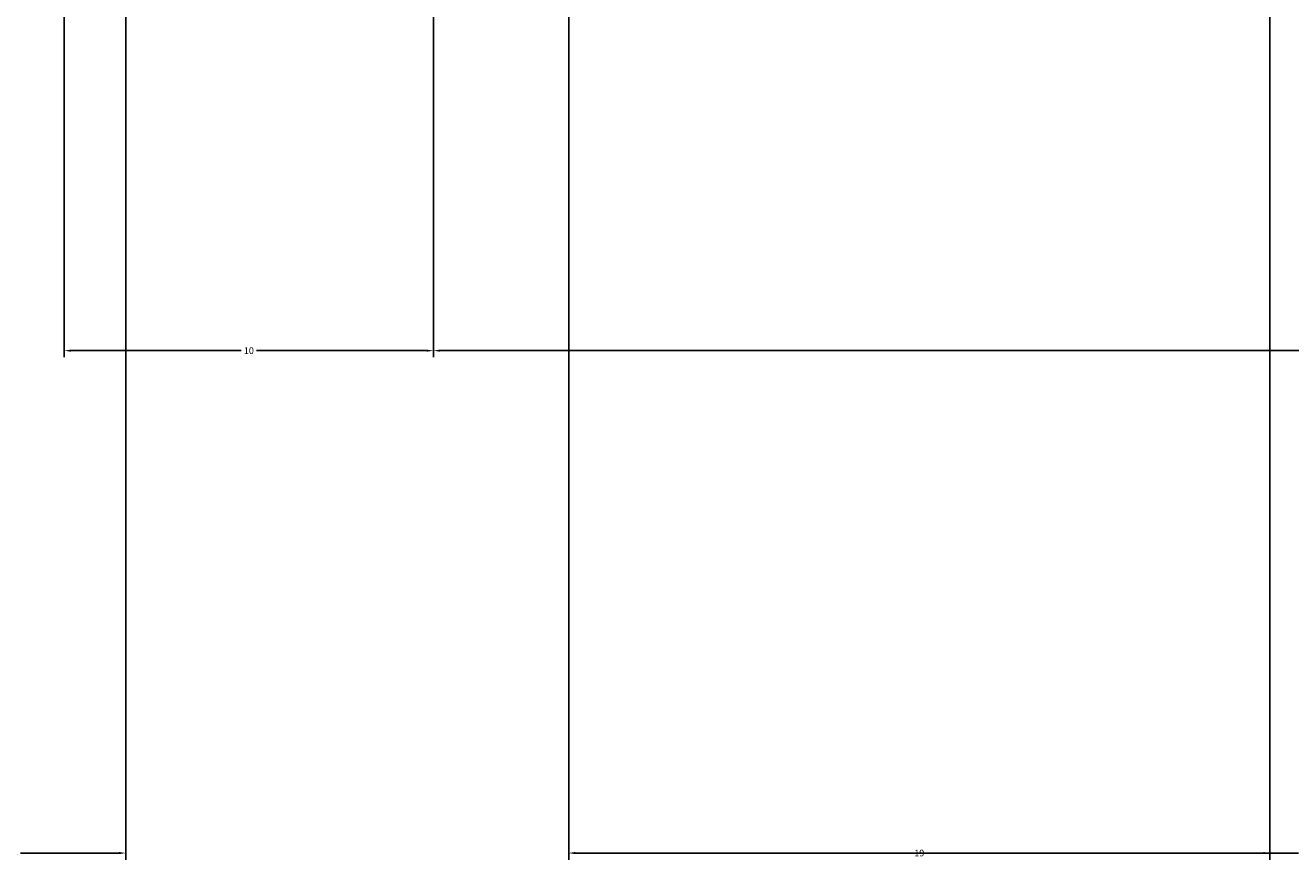
# Model space of a CAD drawing. Units: inches. Extents: x -1 to 292, y -3 to 199.
# Tile 13 of 52: x 68 to 102, y -3 to 20. Entities that reach past the tile are written whole.
import ezdxf

# ---------------------------------------------------------------- set-up
doc = ezdxf.new("R2010")
doc.units = ezdxf.units.IN
doc.header["$MEASUREMENT"] = 0
doc.layers.add('M-DIMS', color=2, linetype='Continuous', lineweight=18)
doc.styles.get("Standard").update_dxf_attribs({"font": 'arial.ttf'})
doc.dimstyles.get("Standard").update_dxf_attribs({"dimtxt": 0.18, "dimasz": 0.18, "dimexe": 0.18, "dimexo": 0.0625, "dimgap": 0.09, "dimtad": 0, "dimtih": 1, "dimtoh": 1, "dimdec": 4, "dimzin": 0, "dimdsep": 46, "dimtxsty": 'Standard', "dimcen": 0.09, "dimadec": 0, "dimazin": 0, "dimtfac": 1, "dimtdec": 4, "dimtofl": 0, "dimtmove": 0, "dimatfit": 3, "dimfxl": 1, "dimtolj": 1, "dimtzin": 0, "dimarcsym": 0})

# ---------------------------------------------------------------- blocks, each defined once
blk = doc.blocks.new('*D12')
at = {"layer": 'Defpoints', "color": 0, "transparency": 16777216}
for p in [(69.013, 25.514), (79.013, 25.514), (69.013, 10.914)]:
    blk.add_point(p, dxfattribs=at)
at = {"layer": 'M-DIMS', "color": 0, "lineweight": -2, "transparency": 16777216}
for p, q in [((69.013, 25.452), (69.013, 10.734)), ((79.013, 25.452), (79.013, 10.734)), ((69.193, 10.914), (73.803, 10.914)), ((78.833, 10.914), (74.223, 10.914))]:
    blk.add_line(p, q, dxfattribs=at)
at = {"layer": 'M-DIMS', "color": 0, "transparency": 16777216}
for points in [[(69.193, 10.944), (69.193, 10.884), (69.013, 10.914)], [(78.833, 10.944), (78.833, 10.884), (79.013, 10.914)]]:
    blk.add_solid(points, dxfattribs=at)
at = {"layer": 'M-DIMS', "color": 0, "transparency": 16777216, "insert": (74.013, 10.914), "char_height": 0.18, "attachment_point": 5}
blk.add_mtext('\\A1;10', dxfattribs=at)
blk = doc.blocks.new('*D13')
at = {"layer": 'Defpoints', "color": 0, "transparency": 16777216}
for p in [(79.013, 25.514), (148.429, 25.514), (79.013, 10.914)]:
    blk.add_point(p, dxfattribs=at)
at = {"layer": 'M-DIMS', "color": 0, "lineweight": -2, "transparency": 16777216}
for p, q in [((79.013, 25.452), (79.013, 10.734)), ((148.429, 25.452), (148.429, 10.734)), ((79.193, 10.914), (113.328, 10.914)), ((148.249, 10.914), (114.115, 10.914))]:
    blk.add_line(p, q, dxfattribs=at)
at = {"layer": 'M-DIMS', "color": 0, "transparency": 16777216}
for points in [[(79.193, 10.944), (79.193, 10.884), (79.013, 10.914)], [(148.249, 10.944), (148.249, 10.884), (148.429, 10.914)]]:
    blk.add_solid(points, dxfattribs=at)
at = {"layer": 'M-DIMS', "color": 0, "transparency": 16777216, "insert": (113.721, 10.914), "char_height": 0.18, "attachment_point": 5}
blk.add_mtext('\\A1;69.42', dxfattribs=at)
blk = doc.blocks.new('*D20')
at = {"layer": 'Defpoints', "color": 0, "transparency": 16777216}
for p in [(64.679, 51.267), (70.679, 51.267), (70.679, -2.71)]:
    blk.add_point(p, dxfattribs=at)
at = {"layer": 'M-DIMS', "color": 0, "lineweight": -2, "transparency": 16777216}
for p, q in [((64.679, 51.205), (64.679, -2.89)), ((70.679, 51.205), (70.679, -2.89)), ((64.859, -2.71), (67.529, -2.71)), ((70.499, -2.71), (67.828, -2.71))]:
    blk.add_line(p, q, dxfattribs=at)
at = {"layer": 'M-DIMS', "color": 0, "transparency": 16777216}
for points in [[(64.859, -2.68), (64.859, -2.74), (64.679, -2.71)], [(70.499, -2.68), (70.499, -2.74), (70.679, -2.71)]]:
    blk.add_solid(points, dxfattribs=at)
at = {"layer": 'M-DIMS', "color": 0, "transparency": 16777216, "insert": (67.679, -2.71), "char_height": 0.18, "attachment_point": 5}
blk.add_mtext('\\A1;6', dxfattribs=at)
blk = doc.blocks.new('*D21')
at = {"layer": 'Defpoints', "color": 0, "transparency": 16777216}
for p in [(82.679, 51.267), (101.679, 51.267), (101.679, -2.71)]:
    blk.add_point(p, dxfattribs=at)
at = {"layer": 'M-DIMS', "color": 0, "lineweight": -2, "transparency": 16777216}
for p, q in [((82.679, 51.205), (82.679, -2.89)), ((101.679, 51.205), (101.679, -2.89)), ((82.859, -2.71), (91.968, -2.71)), ((101.499, -2.71), (92.389, -2.71))]:
    blk.add_line(p, q, dxfattribs=at)
at = {"layer": 'M-DIMS', "color": 0, "transparency": 16777216}
for points in [[(82.859, -2.68), (82.859, -2.74), (82.679, -2.71)], [(101.499, -2.68), (101.499, -2.74), (101.679, -2.71)]]:
    blk.add_solid(points, dxfattribs=at)
at = {"layer": 'M-DIMS', "color": 0, "transparency": 16777216, "insert": (92.179, -2.71), "char_height": 0.18, "attachment_point": 5}
blk.add_mtext('\\A1;19', dxfattribs=at)
blk = doc.blocks.new('*D22')
at = {"layer": 'Defpoints', "color": 0, "transparency": 16777216}
for p in [(82.679, 51.267), (122.679, 51.267), (122.679, -2.71)]:
    blk.add_point(p, dxfattribs=at)
at = {"layer": 'M-DIMS', "color": 0, "lineweight": -2, "transparency": 16777216}
for p, q in [((82.679, 51.205), (82.679, -2.89)), ((122.679, 51.205), (122.679, -2.89)), ((82.859, -2.71), (102.457, -2.71)), ((122.499, -2.71), (102.901, -2.71))]:
    blk.add_line(p, q, dxfattribs=at)
at = {"layer": 'M-DIMS', "color": 0, "transparency": 16777216}
for points in [[(82.859, -2.68), (82.859, -2.74), (82.679, -2.71)], [(122.499, -2.68), (122.499, -2.74), (122.679, -2.71)]]:
    blk.add_solid(points, dxfattribs=at)
at = {"layer": 'M-DIMS', "color": 0, "transparency": 16777216, "insert": (102.679, -2.71), "char_height": 0.18, "attachment_point": 5}
blk.add_mtext('\\A1;40', dxfattribs=at)

msp = doc.modelspace()

# ---------------------------------------------------------------- dimensions: what is measured, and where the dimension line sits
at = {"layer": 'M-DIMS'}
for base, p1, p2, picture, middle in [((70.6788, -2.7104), (64.6788, 51.2672), (70.6788, 51.2672), '*D20', (67.6788, -2.7104)), ((101.6788, -2.7104), (82.6788, 51.2672), (101.6788, 51.2672), '*D21', (92.1788, -2.7104)), ((122.6788, -2.7104), (82.6788, 51.2672), (122.6788, 51.2672), '*D22', (102.6788, -2.7104))]:
    dim = msp.add_linear_dim(base=base, p1=p1, p2=p2, dimstyle='Standard', override={"dimdec": 0, "dimlfac": 1, "dimrnd": 0, "dimzin": 0, "dimdsep": 46, "dimlunit": 2}, dxfattribs=at)
    dim.commit()
    dim.dimension.update_dxf_attribs({"geometry": picture, "text_midpoint": middle})
for base, p1, p2, override, picture, middle in [((69.013, 10.9141), (79.013, 25.5141), (69.013, 25.5141), {"dimdec": 0, "dimlfac": 1, "dimrnd": 0, "dimzin": 0, "dimdsep": 46, "dimlunit": 2}, '*D12', (74.013, 10.9141)), ((79.013, 10.9141), (148.4295, 25.5141), (79.013, 25.5141), {"dimdec": 2, "dimlfac": 1, "dimrnd": 0, "dimzin": 0, "dimdsep": 46, "dimlunit": 2}, '*D13', (113.7212, 10.9141))]:
    dim = msp.add_linear_dim(base=base, p1=p1, p2=p2, angle=180, dimstyle='Standard', override=override, dxfattribs=at)
    dim.commit()
    dim.dimension.update_dxf_attribs({"geometry": picture, "text_midpoint": middle})

doc.saveas('drawing.dxf')
